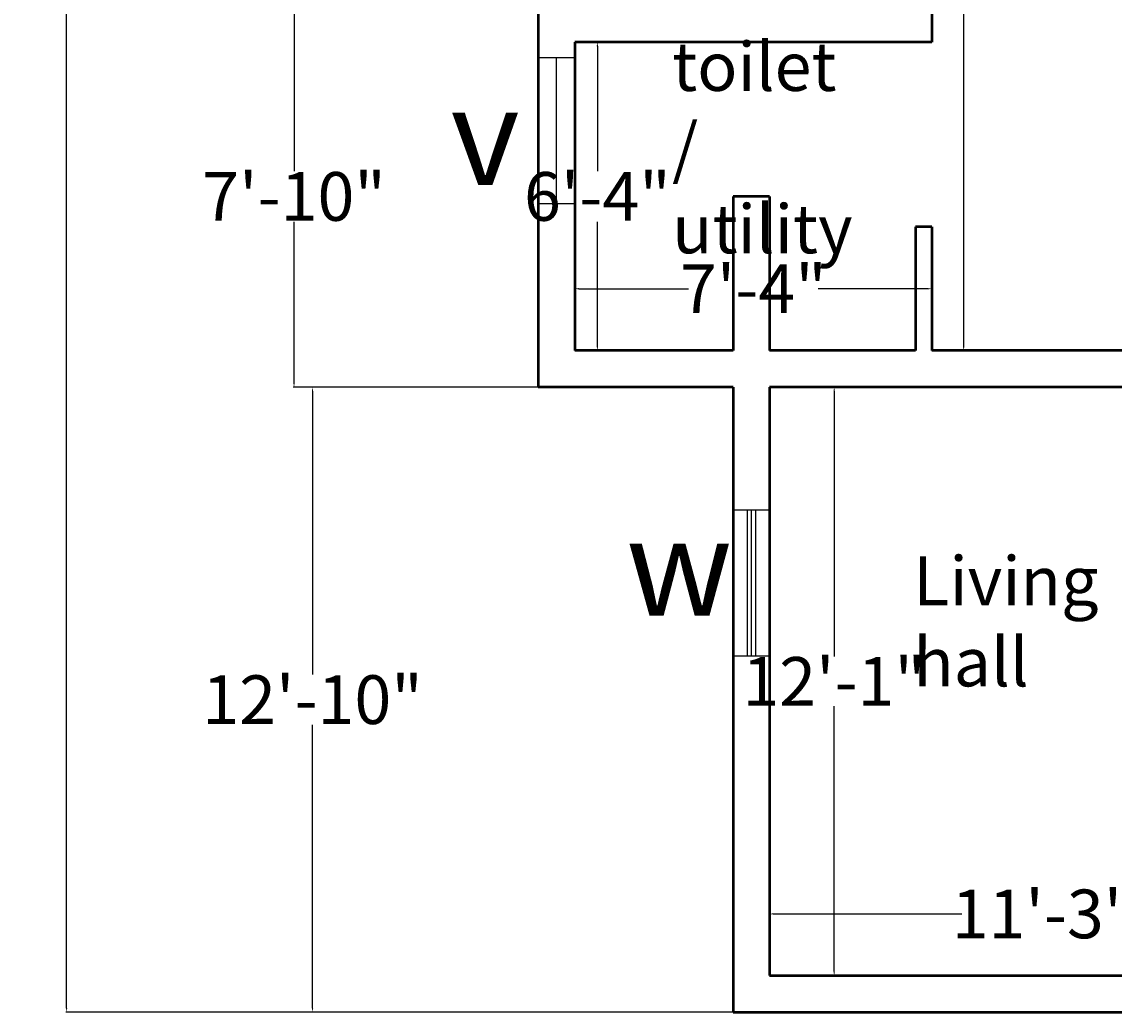
# Model space of a CAD drawing. Units: inches. Extents: x 409 to 7572, y 7 to 725.
# Tile 34 of 38: x 6810 to 7079, y 157 to 401. Entities that reach past the tile are written whole.
import ezdxf

# ---------------------------------------------------------------- set-up
doc = ezdxf.new("R2010")
doc.units = ezdxf.units.IN
doc.header["$MEASUREMENT"] = 0
for name, color, linetype, lineweight in [('A-ANNO-DIMS', 2, 'Continuous', 18), ('A-ANNO-SYMB', 3, 'Continuous', 25), ('A-AREA-IDEN', 7, 'Continuous', 25), ('A-GLAZ', 4, 'Continuous', 25), ('A-WALL', 7, 'Continuous', 50)]:
    doc.layers.add(name, color=color, linetype=linetype, lineweight=lineweight)
doc.styles.get("Standard").update_dxf_attribs({"font": 'arial.ttf'})
doc.dimstyles.get("Standard").update_dxf_attribs({"dimtxt": 2, "dimasz": 1, "dimexe": 0.18, "dimexo": 0.0625, "dimgap": 0.09, "dimtad": 0, "dimtih": 1, "dimtoh": 1, "dimdec": 0, "dimzin": 0, "dimdsep": 46, "dimlunit": 3, "dimtxsty": 'Standard', "dimcen": 0.09, "dimadec": 0, "dimazin": 0, "dimtfac": 1, "dimtdec": 0, "dimtofl": 0, "dimtmove": 0, "dimatfit": 3, "dimfxl": 1, "dimtolj": 1, "dimtzin": 0, "dimarcsym": 0})

# ---------------------------------------------------------------- blocks, each defined once
blk = doc.blocks.new('*D150')
at = {"layer": 'A-ANNO-DIMS', "color": 0, "lineweight": -2, "transparency": 16777216}
for p, q in [((6994.41, 165.59), (6994.41, 180.91)), ((6995.41, 180.73), (7041.78, 180.73)), ((7128.41, 180.73), (7082.05, 180.73)), ((7129.41, 165.59), (7129.41, 180.91))]:
    blk.add_line(p, q, dxfattribs=at)
at = {"layer": 'A-ANNO-DIMS', "color": 0, "transparency": 16777216}
for points in [[(6995.41, 180.9), (6995.41, 180.56), (6994.41, 180.73)], [(7128.41, 180.9), (7128.41, 180.56), (7129.41, 180.73)]]:
    blk.add_solid(points, dxfattribs=at)
at = {"layer": 'DEFPOINTS', "color": 0, "transparency": 16777216}
for p in [(7129.41, 180.73), (6994.41, 165.53), (7129.41, 165.53)]:
    blk.add_point(p, dxfattribs=at)
at = {"layer": 'A-ANNO-DIMS', "color": 0, "transparency": 16777216, "insert": (7061.91, 180.73), "char_height": 2, "attachment_point": 5}
blk.add_mtext('\\A1;{\\H6x;11\'-3"}', dxfattribs=at)
blk = doc.blocks.new('*D151')
at = {"layer": 'A-ANNO-DIMS', "color": 0, "lineweight": -2, "transparency": 16777216}
for p, q in [((6994.47, 310.53), (7010.51, 310.53)), ((7010.33, 309.53), (7010.33, 244.15)), ((7010.33, 166.53), (7010.33, 231.92)), ((6994.47, 165.53), (7010.51, 165.53))]:
    blk.add_line(p, q, dxfattribs=at)
at = {"layer": 'A-ANNO-DIMS', "color": 0, "transparency": 16777216}
for points in [[(7010.17, 309.53), (7010.5, 309.53), (7010.33, 310.53)], [(7010.17, 166.53), (7010.5, 166.53), (7010.33, 165.53)]]:
    blk.add_solid(points, dxfattribs=at)
at = {"layer": 'DEFPOINTS', "color": 0, "transparency": 16777216}
for p in [(6994.41, 310.53), (6994.41, 165.53), (7010.33, 165.53)]:
    blk.add_point(p, dxfattribs=at)
at = {"layer": 'A-ANNO-DIMS', "color": 0, "transparency": 16777216, "insert": (7010.33, 238.03), "char_height": 2, "attachment_point": 5}
blk.add_mtext('\\A1;{\\H6x;12\'-1"}', dxfattribs=at)
blk = doc.blocks.new('*D158')
at = {"layer": 'A-ANNO-DIMS', "color": 0, "lineweight": -2, "transparency": 16777216}
for p, q in [((7051.35, 525.53), (7042.07, 525.53)), ((7042.25, 524.53), (7042.25, 428.65)), ((7042.25, 320.53), (7042.25, 416.42)), ((7059.35, 319.53), (7042.07, 319.53))]:
    blk.add_line(p, q, dxfattribs=at)
at = {"layer": 'A-ANNO-DIMS', "color": 0, "transparency": 16777216}
for points in [[(7042.08, 524.53), (7042.42, 524.53), (7042.25, 525.53)], [(7042.08, 320.53), (7042.42, 320.53), (7042.25, 319.53)]]:
    blk.add_solid(points, dxfattribs=at)
at = {"layer": 'DEFPOINTS', "color": 0, "transparency": 16777216}
for p in [(7051.41, 525.53), (7042.25, 319.53), (7059.41, 319.53)]:
    blk.add_point(p, dxfattribs=at)
at = {"layer": 'A-ANNO-DIMS', "color": 0, "transparency": 16777216, "insert": (7042.25, 422.53), "char_height": 2, "attachment_point": 5}
blk.add_mtext('\\A1;{\\H6x;17\'-2"}', dxfattribs=at)
blk = doc.blocks.new('*D159')
at = {"layer": 'A-ANNO-DIMS', "color": 0, "lineweight": -2, "transparency": 16777216}
for p, q in [((6955.62, 395.53), (6951.79, 395.53)), ((6951.97, 394.53), (6951.97, 363.75)), ((6951.97, 320.53), (6951.97, 351.31)), ((6955.62, 319.53), (6951.79, 319.53))]:
    blk.add_line(p, q, dxfattribs=at)
at = {"layer": 'A-ANNO-DIMS', "color": 0, "transparency": 16777216}
for points in [[(6951.81, 394.53), (6952.14, 394.53), (6951.97, 395.53)], [(6951.81, 320.53), (6952.14, 320.53), (6951.97, 319.53)]]:
    blk.add_solid(points, dxfattribs=at)
at = {"layer": 'DEFPOINTS', "color": 0, "transparency": 16777216}
for p in [(6955.68, 395.53), (6951.97, 319.53), (6955.68, 319.53)]:
    blk.add_point(p, dxfattribs=at)
at = {"layer": 'A-ANNO-DIMS', "color": 0, "transparency": 16777216, "insert": (6951.97, 357.53), "char_height": 2, "attachment_point": 5}
blk.add_mtext('\\A1;{\\H6x;6\'-4"}', dxfattribs=at)
blk = doc.blocks.new('*D160')
at = {"layer": 'A-ANNO-DIMS', "color": 0, "lineweight": -2, "transparency": 16777216}
for p, q in [((6946.41, 346.33), (6946.41, 334.6)), ((7034.41, 346.33), (7034.41, 334.6)), ((6947.41, 334.78), (6974.42, 334.78)), ((7033.41, 334.78), (7006.4, 334.78))]:
    blk.add_line(p, q, dxfattribs=at)
at = {"layer": 'A-ANNO-DIMS', "color": 0, "transparency": 16777216}
for points in [[(6947.41, 334.95), (6947.41, 334.61), (6946.41, 334.78)], [(7033.41, 334.95), (7033.41, 334.61), (7034.41, 334.78)]]:
    blk.add_solid(points, dxfattribs=at)
at = {"layer": 'DEFPOINTS', "color": 0, "transparency": 16777216}
for p in [(6946.41, 346.39), (7034.41, 346.39), (7034.41, 334.78)]:
    blk.add_point(p, dxfattribs=at)
at = {"layer": 'A-ANNO-DIMS', "color": 0, "transparency": 16777216, "insert": (6990.41, 334.78), "char_height": 2, "attachment_point": 5}
blk.add_mtext('\\A1;{\\H6x;7\'-4"}', dxfattribs=at)
blk = doc.blocks.new('*D155')
at = {"layer": 'A-ANNO-DIMS', "color": 0, "lineweight": -2, "transparency": 16777216}
for p, q in [((6937.35, 404.53), (6877.04, 404.53)), ((6877.22, 403.53), (6877.22, 363.75)), ((6877.22, 311.53), (6877.22, 351.31)), ((6937.35, 310.53), (6877.04, 310.53))]:
    blk.add_line(p, q, dxfattribs=at)
at = {"layer": 'A-ANNO-DIMS', "color": 0, "transparency": 16777216}
for points in [[(6877.05, 403.53), (6877.39, 403.53), (6877.22, 404.53)], [(6877.05, 311.53), (6877.39, 311.53), (6877.22, 310.53)]]:
    blk.add_solid(points, dxfattribs=at)
at = {"layer": 'DEFPOINTS', "color": 0, "transparency": 16777216}
for p in [(6937.41, 404.53), (6877.22, 310.53), (6937.41, 310.53)]:
    blk.add_point(p, dxfattribs=at)
at = {"layer": 'A-ANNO-DIMS', "color": 0, "transparency": 16777216, "insert": (6877.22, 357.53), "char_height": 2, "attachment_point": 5}
blk.add_mtext('\\A1;{\\H6x;7\'-10"}', dxfattribs=at)
blk = doc.blocks.new('*D156')
at = {"layer": 'A-ANNO-DIMS', "color": 0, "lineweight": -2, "transparency": 16777216}
for p, q in [((6985.35, 310.53), (6881.6, 310.53)), ((6881.78, 309.53), (6881.78, 239.75)), ((6881.78, 157.53), (6881.78, 227.31)), ((6985.35, 156.53), (6881.6, 156.53))]:
    blk.add_line(p, q, dxfattribs=at)
at = {"layer": 'A-ANNO-DIMS', "color": 0, "transparency": 16777216}
for points in [[(6881.62, 309.53), (6881.95, 309.53), (6881.78, 310.53)], [(6881.62, 157.53), (6881.95, 157.53), (6881.78, 156.53)]]:
    blk.add_solid(points, dxfattribs=at)
at = {"layer": 'DEFPOINTS', "color": 0, "transparency": 16777216}
for p in [(6985.41, 310.53), (6881.78, 156.53), (6985.41, 156.53)]:
    blk.add_point(p, dxfattribs=at)
at = {"layer": 'A-ANNO-DIMS', "color": 0, "transparency": 16777216, "insert": (6881.78, 233.53), "char_height": 2, "attachment_point": 5}
blk.add_mtext('\\A1;{\\H6x;12\'-10"}', dxfattribs=at)
blk = doc.blocks.new('*D149')
at = {"layer": 'A-ANNO-DIMS', "color": 0, "lineweight": -2, "transparency": 16777216}
for p, q in [((6985.35, 672.53), (6820.99, 672.53)), ((6821.17, 671.53), (6821.17, 420.75)), ((6821.17, 157.53), (6821.17, 408.31)), ((6985.35, 156.53), (6820.99, 156.53))]:
    blk.add_line(p, q, dxfattribs=at)
at = {"layer": 'A-ANNO-DIMS', "color": 0, "transparency": 16777216}
for points in [[(6821.01, 671.53), (6821.34, 671.53), (6821.17, 672.53)], [(6821.01, 157.53), (6821.34, 157.53), (6821.17, 156.53)]]:
    blk.add_solid(points, dxfattribs=at)
at = {"layer": 'DEFPOINTS', "color": 0, "transparency": 16777216}
for p in [(6985.41, 672.53), (6821.17, 156.53), (6985.41, 156.53)]:
    blk.add_point(p, dxfattribs=at)
at = {"layer": 'A-ANNO-DIMS', "color": 0, "transparency": 16777216, "insert": (6821.17, 414.53), "char_height": 2, "attachment_point": 5}
blk.add_mtext("\\A1;{\\H6x;43'}", dxfattribs=at)
blk = doc.blocks.new('WIN-36')
for p, q in [((1699.82, 514.65), (1699.82, 478.65)), ((1700.82, 514.65), (1700.82, 478.65)), ((1701.82, 514.65), (1701.82, 478.65))]:
    blk.add_line(p, q)
blk.add_lwpolyline([(1705.32, 514.65), (1705.32, 478.65), (1696.32, 478.65), (1696.32, 514.65)], close=True)
blk = doc.blocks.new('VENT-36')
blk.add_line((5633.28, 355.73), (5633.28, 391.73))
blk.add_lwpolyline([(5628.78, 355.73), (5628.78, 391.73), (5637.78, 391.73), (5637.78, 355.73)], close=True)

msp = doc.modelspace()

# ---------------------------------------------------------------- linework, layer by layer
at = {"layer": 'A-WALL'}
for p, q in [((6937.41, 404.53), (6937.41, 310.53)), ((7034.41, 404.53), (7034.41, 395.53)), ((6994.41, 395.53), (6946.41, 395.53)), ((6946.41, 395.53), (6946.41, 319.53)), ((7034.41, 395.53), (6994.41, 395.53)), ((6985.41, 357.53), (6985.41, 319.53)), ((6994.41, 357.53), (6985.41, 357.53)), ((6994.41, 357.53), (6994.41, 319.53)), ((7030.41, 350.03), (7030.41, 319.53)), ((7034.41, 350.03), (7030.41, 350.03)), ((7034.41, 350.03), (7034.41, 319.53)), ((6985.41, 319.53), (6946.41, 319.53)), ((7030.41, 319.53), (6994.41, 319.53)), ((7084.41, 319.53), (7034.41, 319.53)), ((6985.41, 310.53), (6937.41, 310.53)), ((6985.41, 310.53), (6985.41, 156.53)), ((7084.41, 310.53), (6994.41, 310.53)), ((6994.41, 310.53), (6994.41, 165.53)), ((6994.41, 165.53), (7129.41, 165.53)), ((6985.41, 156.53), (7359.41, 156.53))]:
    msp.add_line(p, q, dxfattribs=at)

# ---------------------------------------------------------------- block references
at = {"layer": 'A-GLAZ'}
for name, p in [('VENT-36', (1308.63, 0)), ('WIN-36', (5289.09, -234.38))]:
    msp.add_blockref(name, p, dxfattribs=at)

# ---------------------------------------------------------------- texts
at = {"layer": 'A-ANNO-SYMB', "char_height": 24, "attachment_point": 1}
for s, insert in [('v', (6915.77, 384.37)), ('w', (6959, 278.21))]:
    msp.add_mtext_dynamic_manual_height_columns(s, width=18.2582, gutter_width=1, heights=[0], dxfattribs=dict(at, insert=insert))
at = {"layer": 'A-AREA-IDEN', "char_height": 12, "attachment_point": 1}
for s, width, insert in [('toilet / utility', 49.2946, (6970.41, 395.53)), ('Living hall', 58.8843, (7029.84, 268.81))]:
    msp.add_mtext_dynamic_manual_height_columns(s, width=width, gutter_width=1, heights=[0], dxfattribs=dict(at, insert=insert))

# ---------------------------------------------------------------- dimensions: what is measured, and where the dimension line sits
at = {"layer": 'A-ANNO-DIMS'}
for base, p1, p2, picture, middle in [((6821.17, 156.53), (6985.41, 672.53), (6985.41, 156.53), '*D149', (6821.17, 414.53)), ((6877.22, 310.53), (6937.41, 404.53), (6937.41, 310.53), '*D155', (6877.22, 357.53)), ((6951.97, 319.53), (6955.68, 395.53), (6955.68, 319.53), '*D159', (6951.97, 357.53)), ((6881.78, 156.53), (6985.41, 310.53), (6985.41, 156.53), '*D156', (6881.78, 233.53)), ((7010.33, 165.53), (6994.41, 310.53), (6994.41, 165.53), '*D151', (7010.33, 238.03))]:
    dim = msp.add_linear_dim(base=base, p1=p1, p2=p2, angle=90, text='{\\H6x;<>}', dimstyle='Standard', override={"dimclrd": 0, "dimclre": 0, "dimclrt": 0}, dxfattribs=at)
    dim.commit()
    dim.dimension.update_dxf_attribs({"geometry": picture, "text_midpoint": middle})
dim = msp.add_linear_dim(base=(7042.25, 319.53), p1=(7051.41, 525.53), p2=(7059.41, 319.53), angle=90, text='{\\H6x;<>}', dimstyle='Standard', override={"dimclrd": 0, "dimclre": 0, "dimclrt": 0}, dxfattribs=at)
dim.commit()
dim.dimension.update_dxf_attribs({"geometry": '*D158', "text_midpoint": (7042.25, 422.53), "dimtype": 160})
for base, p1, p2, picture, middle in [((7034.41, 334.78), (6946.41, 346.39), (7034.41, 346.39), '*D160', (6990.41, 334.78)), ((7129.41, 180.73), (6994.41, 165.53), (7129.41, 165.53), '*D150', (7061.91, 180.73))]:
    dim = msp.add_linear_dim(base=base, p1=p1, p2=p2, text='{\\H6x;<>}', dimstyle='Standard', override={"dimclrd": 0, "dimclre": 0, "dimclrt": 0}, dxfattribs=at)
    dim.commit()
    dim.dimension.update_dxf_attribs({"geometry": picture, "text_midpoint": middle})

doc.saveas('drawing.dxf')
